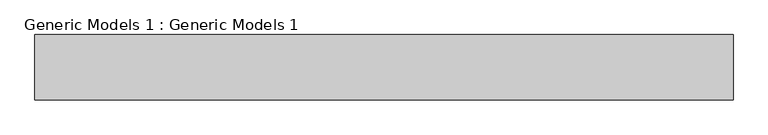
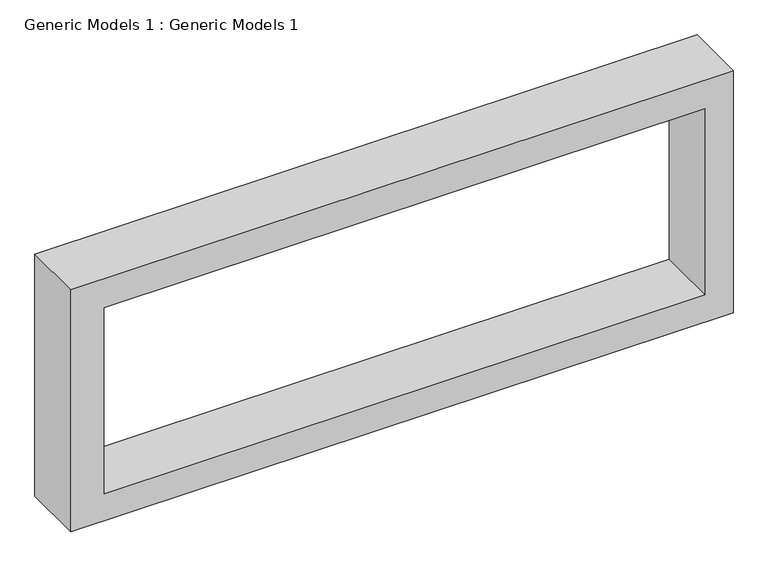
"""IFC4 building model written with IfcOpenShell, lengths in millimetres: proxy geometry, Generic Models 1 : Generic Models 1."""

from ifc_helpers import new_model, si_unit, frame, origin, place, context, project, spatial, polyline, outline, extrude, source, transform, mapped, element, save


def generic_models_1_generic_models_1_5f3879a5(model_context):
    return source(origin(), model_context, "Body", "SweptSolid", [
        extrude(outline(polyline([(1566.4444449, -3402.9305709), (1566.4444449, -6650.9555709), (311.8998071, -6650.9555709), (311.8998071, -3402.9305709), (1566.4444449, -3402.9305709)]), holes=[polyline([(1417.4040427, -3541.0240901), (452.2040427, -3541.0240901), (452.2040427, -6487.4240901), (1417.4040427, -6487.4240901), (1417.4040427, -3541.0240901)])]), frame((0.0, -7272.3064015, 0.0), z_axis=(0.0, 1.0, 0.0), x_axis=(0.0, 0.0, 1.0)), (0.0, 0.0, 1.0), 304.8),
    ])


if __name__ == "__main__":
    model = new_model("IFC4")
    model_context = context("Model", 3, world=origin())
    ifc_project = project(units=[si_unit("LENGTHUNIT", "METRE", prefix="MILLI")], contexts=[model_context])
    site = spatial("IfcSite", under=ifc_project)
    building = spatial("IfcBuilding", under=site)
    placement = place(None, origin())
    generic_models_1_generic_models_1_shape = generic_models_1_generic_models_1_5f3879a5(model_context)
    element("IfcBuildingElementProxy", 1, Name="Generic Models 1 : Generic Models 1", ObjectType="Generic Models 1 : Generic Models 1", at=placement, inside=building, context=model_context, shape_type="MappedRepresentation", body=[
        mapped(generic_models_1_generic_models_1_shape, transform((0.0, 0.0, 0.0), x_axis=(1.0, 0.0, 0.0), y_axis=(0.0, 1.0, 0.0), z_axis=(0.0, 0.0, 1.0))),
    ])
    save(model, "model.ifc")

# Revit data of these elements
# Element 1 (IfcBuildingElementProxy, "Generic Models 1 : Generic Models 1")
#   Materials on its faces: "Parking Stripe"
# Materials
#   "Parking Stripe": class "Paint", colour RGB 250 250 91, transparency 0, Cost = 0
